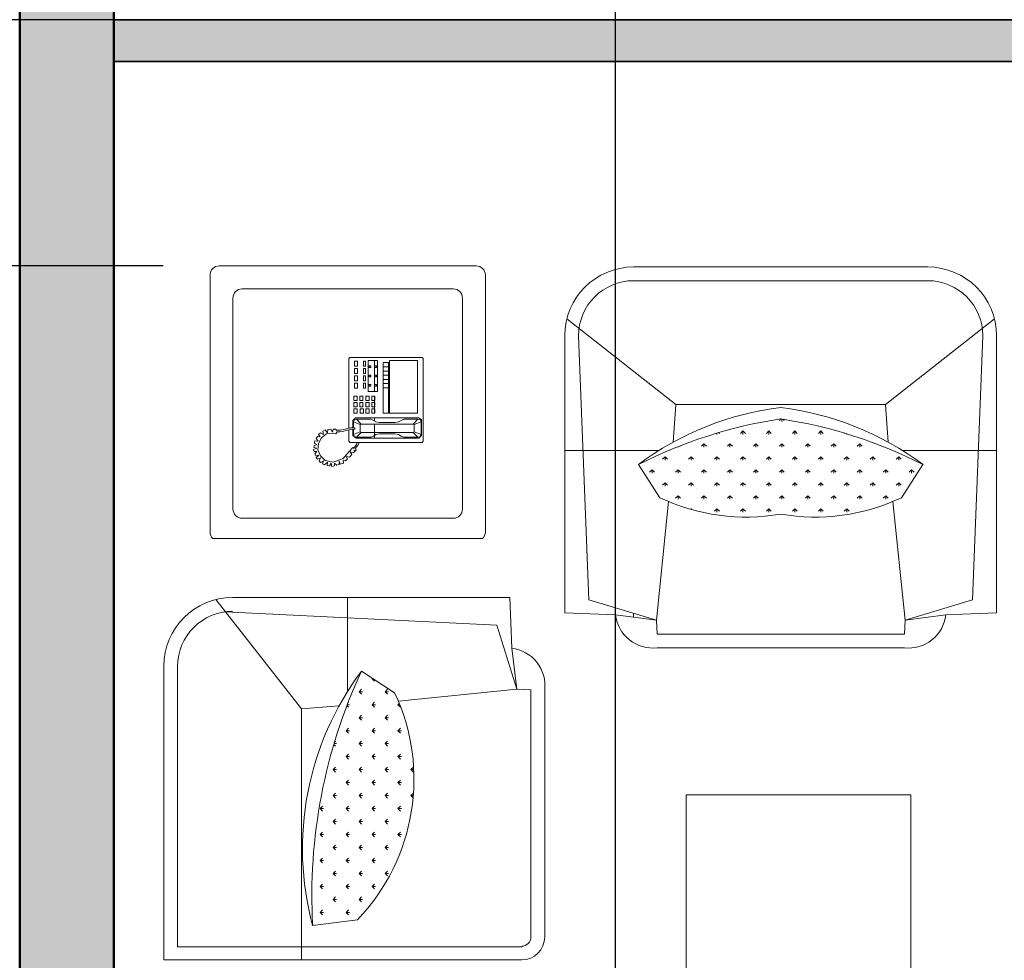
# Model space of a CAD drawing. Units: inches. Extents: x 2796 to 3603, y 978 to 1787.
# Tile 4 of 15: x 3070 to 3165, y 1222 to 1312. Entities that reach past the tile are written whole.
import ezdxf

# ---------------------------------------------------------------- set-up
doc = ezdxf.new("R2010")
doc.units = ezdxf.units.IN
for name, color, linetype, lineweight in [('A-ANNO-DIMS', 7, 'Continuous', 18), ('A-WALL-EXTR-PATT', 1, 'Continuous', 13), ('A-WALL-INTR-PATT', 5, 'Continuous', 13), ('Furniture', 2, 'Continuous', 18), ('Inner Wall', 5, 'Continuous', 35), ('Outer Wall', 1, 'Continuous', 50)]:
    doc.layers.add(name, color=color, linetype=linetype, lineweight=lineweight)
doc.styles.get("Standard").update_dxf_attribs({"font": 'arial.ttf'})
doc.dimstyles.get("Standard").update_dxf_attribs({"dimtxt": 18, "dimasz": 12, "dimexe": 0.18, "dimexo": 0.0625, "dimgap": 0.09, "dimtad": 0, "dimtih": 1, "dimtoh": 1, "dimdec": 0, "dimzin": 0, "dimdsep": 46, "dimlunit": 3, "dimtxsty": 'Standard', "dimcen": 0.09, "dimadec": 0, "dimazin": 0, "dimtfac": 1, "dimtdec": 0, "dimtofl": 0, "dimtmove": 0, "dimatfit": 3, "dimfxl": 1, "dimtolj": 1, "dimtzin": 0, "dimarcsym": 0})

# ---------------------------------------------------------------- blocks, each defined once
blk = doc.blocks.new('A$C16A87060')
at = {"ltscale": 2}
for p, q in [((272, 1415.3), (103.9, 1629.3)), ((362, 1633.4), (362, 1448.5)), ((137, 1606.4), (655.3, 1586)), ((655.3, 1586), (694.6, 1453.8)), ((684.3, 1533.8), (694.6, 1453.8)), ((29, 1498.4), (29, 1209.9)), ((389.7, 1489), (454.7, 1446.7)), ((694.6, 1453.8), (462.1, 1430.1)), ((722, 1452.4), (694.6, 1453.8)), ((722, 1209.9), (722, 1452.4)), ((345.9, 1421), (272, 1415.3)), ((272, 1415.3), (272, 1209.9)), ((29, 921.4), (29, 1209.9)), ((272, 1004.5), (272, 1209.9)), ((722, 1209.9), (722, 967.4)), ((272, 1004.5), (103.9, 790.5)), ((345.9, 998.8), (272, 1004.5)), ((694.6, 966), (462.1, 989.7)), ((362, 786.4), (362, 971.3)), ((389.7, 930.8), (454.7, 973.1)), ((655.3, 833.8), (694.6, 966)), ((684.3, 886), (694.6, 966)), ((722, 967.4), (694.6, 966)), ((137, 813.4), (655.3, 833.8))]:
    blk.add_line(p, q, dxfattribs=at)
for p, q in [((680.7, 1633.4), (137, 1633.4)), ((684.3, 1533.8), (680.7, 1633.4)), ((2, 1498.4), (2, 1209.9)), ((749, 1209.9), (749, 1452.4)), ((1037.3, 1465.2), (2216.9, 1465.2)), ((1037.3, 1024.2), (1037.3, 1465.2)), ((2, 921.4), (2, 1209.9)), ((749, 1209.9), (749, 967.4)), ((2216.9, 1024.2), (1037.3, 1024.2)), ((681.3, 921.3), (688.8, 921.3)), ((684.3, 886), (680.7, 786.4)), ((680.7, 786.4), (137, 786.4)), ((1316.4, 747), (831.4, 747)), ((831.4, 720), (830, 692.5)), ((1316.4, 720), (831.4, 720)), ((1335.7, 27), (1335.7, 702.9)), ((1361.4, 702), (1361.4, 0)), ((750, 682.3), (650.4, 678.6)), ((650.4, 678.6), (650.4, 135)), ((704.4, 653.3), (830, 692.5)), ((750, 682.3), (830, 692.5)), ((830, 692.5), (853.7, 460)), ((678.3, 120.6), (704.4, 653.3)), ((18, 630.6), (522, 630.6)), ((534.7, 625.3), (534.7, 95.9)), ((0, 108.6), (0, 612.6)), ((63, 585.6), (477, 585.6)), ((45, 153.6), (45, 567.6)), ((495, 567.6), (495, 153.6)), ((794.8, 387.7), (837.1, 452.7)), ((185.6, 413.3), (246.3, 413.3)), ((255.5, 413.3), (288.5, 413.3)), ((297.7, 413.3), (304.3, 413.3)), ((310.1, 413.3), (332.3, 413.3)), ((332.3, 413.3), (337.8, 413.3)), ((1282.5, 379.8), (1294.1, 291.9)), ((650.4, 360), (835.3, 360)), ((862.8, 343.9), (868.5, 270)), ((868.5, 270), (654.5, 101.9)), ((868.5, 270), (1361.4, 270)), ((477, 135.6), (63, 135.6)), ((522, 90.6), (18, 90.6)), ((785.4, 27), (1335.7, 27)), ((785.4, 0), (1361.4, 0))]:
    blk.add_line(p, q)
at = {"linetype": 'ByBlock'}
for p, q in [((400, 1466.7), (404.7, 1471.5)), ((400, 1466.7), (406.7, 1466.7)), ((400, 1466.7), (404.7, 1462)), ((374.5, 1441.3), (379.3, 1446.1)), ((374.5, 1441.3), (381.3, 1441.3)), ((374.5, 1441.3), (379.3, 1436.5)), ((425.4, 1441.3), (430.2, 1446.1)), ((425.4, 1441.3), (432.2, 1441.3)), ((425.4, 1441.3), (430.2, 1436.5)), ((400, 1415.8), (404.7, 1420.6)), ((400, 1415.8), (406.7, 1415.8)), ((400, 1415.8), (404.7, 1411.1)), ((450.9, 1415.8), (455.7, 1420.6)), ((450.9, 1415.8), (457.6, 1415.8)), ((450.9, 1415.8), (455.7, 1411.1)), ((374.5, 1390.4), (379.3, 1395.1)), ((425.4, 1390.4), (430.2, 1395.1)), ((374.5, 1390.4), (381.3, 1390.4)), ((374.5, 1390.4), (379.3, 1385.6)), ((425.4, 1390.4), (432.2, 1390.4)), ((425.4, 1390.4), (430.2, 1385.6)), ((349.1, 1364.9), (353.8, 1369.7)), ((349.1, 1364.9), (355.8, 1364.9)), ((349.1, 1364.9), (353.8, 1360.1)), ((400, 1364.9), (404.7, 1369.7)), ((400, 1364.9), (406.7, 1364.9)), ((400, 1364.9), (404.7, 1360.1)), ((450.9, 1364.9), (455.7, 1369.7)), ((450.9, 1364.9), (457.6, 1364.9)), ((450.9, 1364.9), (455.7, 1360.1)), ((328, 1335.1), (328.4, 1334.7)), ((329.3, 1339.5), (330.4, 1339.5)), ((374.5, 1339.5), (379.3, 1344.2)), ((374.5, 1339.5), (381.3, 1339.5)), ((374.5, 1339.5), (379.3, 1334.7)), ((425.4, 1339.5), (430.2, 1344.2)), ((425.4, 1339.5), (432.2, 1339.5)), ((425.4, 1339.5), (430.2, 1334.7)), ((476.3, 1339.5), (481.1, 1344.2)), ((476.3, 1339.5), (483.1, 1339.5)), ((476.3, 1339.5), (481.1, 1334.7)), ((349.1, 1314), (353.8, 1318.8)), ((349.1, 1314), (355.8, 1314)), ((349.1, 1314), (353.8, 1309.2)), ((400, 1314), (404.7, 1318.8)), ((400, 1314), (406.7, 1314)), ((400, 1314), (404.7, 1309.2)), ((450.9, 1314), (455.7, 1318.8)), ((450.9, 1314), (457.6, 1314)), ((450.9, 1314), (455.7, 1309.2)), ((323.6, 1288.5), (328.4, 1293.3)), ((323.6, 1288.5), (330.4, 1288.5)), ((323.6, 1288.5), (328.4, 1283.8)), ((374.5, 1288.5), (379.3, 1293.3)), ((374.5, 1288.5), (381.3, 1288.5)), ((374.5, 1288.5), (379.3, 1283.8)), ((425.4, 1288.5), (430.2, 1293.3)), ((425.4, 1288.5), (432.2, 1288.5)), ((425.4, 1288.5), (430.2, 1283.8)), ((476.3, 1288.5), (481.1, 1293.3)), ((476.3, 1288.5), (483.1, 1288.5)), ((476.3, 1288.5), (481.1, 1283.8)), ((349.1, 1263.1), (353.8, 1267.9)), ((349.1, 1263.1), (355.8, 1263.1)), ((349.1, 1263.1), (353.8, 1258.3)), ((400, 1263.1), (404.7, 1267.9)), ((400, 1263.1), (406.7, 1263.1)), ((400, 1263.1), (404.7, 1258.3)), ((450.9, 1263.1), (455.7, 1267.9)), ((450.9, 1263.1), (457.6, 1263.1)), ((450.9, 1263.1), (455.7, 1258.3)), ((323.6, 1237.6), (328.4, 1242.4)), ((323.6, 1237.6), (330.4, 1237.6)), ((323.6, 1237.6), (328.4, 1232.9)), ((374.5, 1237.6), (379.3, 1242.4)), ((374.5, 1237.6), (381.3, 1237.6)), ((374.5, 1237.6), (379.3, 1232.9)), ((425.4, 1237.6), (430.2, 1242.4)), ((425.4, 1237.6), (432.2, 1237.6)), ((425.4, 1237.6), (430.2, 1232.9)), ((476.3, 1237.6), (481.1, 1242.4)), ((476.3, 1237.6), (483.1, 1237.6)), ((476.3, 1237.6), (481.1, 1232.9)), ((300.8, 1214.8), (302.9, 1216.9)), ((349.1, 1212.2), (353.8, 1216.9)), ((400, 1212.2), (404.7, 1216.9)), ((450.9, 1212.2), (455.7, 1216.9)), ((300.1, 1210.2), (302.9, 1207.4)), ((300.4, 1212.2), (304.9, 1212.2)), ((349.1, 1212.2), (355.8, 1212.2)), ((349.1, 1212.2), (353.8, 1207.4)), ((400, 1212.2), (406.7, 1212.2)), ((400, 1212.2), (404.7, 1207.4)), ((450.9, 1212.2), (457.6, 1212.2)), ((450.9, 1212.2), (455.7, 1207.4)), ((323.6, 1186.7), (328.4, 1191.5)), ((323.6, 1186.7), (330.4, 1186.7)), ((323.6, 1186.7), (328.4, 1181.9)), ((374.5, 1186.7), (379.3, 1191.5)), ((374.5, 1186.7), (381.3, 1186.7)), ((374.5, 1186.7), (379.3, 1181.9)), ((425.4, 1186.7), (430.2, 1191.5)), ((425.4, 1186.7), (432.2, 1186.7)), ((425.4, 1186.7), (430.2, 1181.9)), ((476.3, 1186.7), (481.1, 1191.5)), ((476.3, 1186.7), (483.1, 1186.7)), ((476.3, 1186.7), (481.1, 1181.9)), ((349.1, 1161.3), (353.8, 1166)), ((349.1, 1161.3), (355.8, 1161.3)), ((349.1, 1161.3), (353.8, 1156.5)), ((400, 1161.3), (404.7, 1166)), ((400, 1161.3), (406.7, 1161.3)), ((400, 1161.3), (404.7, 1156.5)), ((450.9, 1161.3), (455.7, 1166)), ((450.9, 1161.3), (457.6, 1161.3)), ((450.9, 1161.3), (455.7, 1156.5)), ((323.6, 1135.8), (328.4, 1140.6)), ((374.5, 1135.8), (379.3, 1140.6)), ((425.4, 1135.8), (430.2, 1140.6)), ((476.3, 1135.8), (481.1, 1140.6)), ((323.6, 1135.8), (330.4, 1135.8)), ((323.6, 1135.8), (328.4, 1131)), ((374.5, 1135.8), (381.3, 1135.8)), ((374.5, 1135.8), (379.3, 1131)), ((425.4, 1135.8), (432.2, 1135.8)), ((425.4, 1135.8), (430.2, 1131)), ((476.3, 1135.8), (483.1, 1135.8)), ((476.3, 1135.8), (481.1, 1131)), ((349.1, 1110.4), (353.8, 1115.1)), ((349.1, 1110.4), (355.8, 1110.4)), ((349.1, 1110.4), (353.8, 1105.6)), ((400, 1110.4), (404.7, 1115.1)), ((400, 1110.4), (406.7, 1110.4)), ((400, 1110.4), (404.7, 1105.6)), ((450.9, 1110.4), (455.7, 1115.1)), ((450.9, 1110.4), (457.6, 1110.4)), ((450.9, 1110.4), (455.7, 1105.6)), ((327, 1088.2), (328.4, 1089.7)), ((327.9, 1084.9), (330.4, 1084.9)), ((374.5, 1084.9), (379.3, 1089.7)), ((374.5, 1084.9), (381.3, 1084.9)), ((374.5, 1084.9), (379.3, 1080.1)), ((425.4, 1084.9), (430.2, 1089.7)), ((425.4, 1084.9), (432.2, 1084.9)), ((425.4, 1084.9), (430.2, 1080.1)), ((476.3, 1084.9), (481.1, 1089.7)), ((476.3, 1084.9), (483.1, 1084.9)), ((476.3, 1084.9), (481.1, 1080.1)), ((349.1, 1059.4), (353.8, 1064.2)), ((400, 1059.4), (404.7, 1064.2)), ((450.9, 1059.4), (455.7, 1064.2)), ((349.1, 1059.4), (355.8, 1059.4)), ((349.1, 1059.4), (353.8, 1054.7)), ((400, 1059.4), (406.7, 1059.4)), ((400, 1059.4), (404.7, 1054.7)), ((450.9, 1059.4), (457.6, 1059.4)), ((450.9, 1059.4), (455.7, 1054.7)), ((374.5, 1034), (379.3, 1038.8)), ((374.5, 1034), (381.3, 1034)), ((374.5, 1034), (379.3, 1029.2)), ((425.4, 1034), (430.2, 1038.8)), ((425.4, 1034), (432.2, 1034)), ((425.4, 1034), (430.2, 1029.2)), ((476.3, 1034), (478, 1035.6)), ((476.3, 1034), (477.5, 1034)), ((476.3, 1034), (477.2, 1033.1)), ((352.9, 1012.4), (353.8, 1013.3)), ((354.5, 1008.5), (355.8, 1008.5)), ((400, 1008.5), (404.7, 1013.3)), ((400, 1008.5), (406.7, 1008.5)), ((400, 1008.5), (404.7, 1003.8)), ((450.9, 1008.5), (455.7, 1013.3)), ((450.9, 1008.5), (457.6, 1008.5)), ((450.9, 1008.5), (455.7, 1003.8)), ((374.5, 983.1), (379.3, 987.8)), ((425.4, 983.1), (430.2, 987.8)), ((374.5, 983.1), (381.3, 983.1)), ((374.5, 983.1), (379.3, 978.3)), ((425.4, 983.1), (432.2, 983.1)), ((425.4, 983.1), (430.2, 978.3)), ((400, 957.6), (404.7, 962.4)), ((400, 957.6), (406.7, 957.6)), ((400, 957.6), (404.7, 952.8)), ((181.5, 508.6), (179.4, 506.6)), ((179.4, 506.6), (179.4, 364.6)), ((181.5, 508.6), (344, 508.6)), ((297.7, 500.4), (301.8, 505.5)), ((301.8, 502.5), (300.8, 498.3)), ((301.8, 505.5), (332.7, 505.5)), ((306, 504.5), (301.8, 502.5)), ((311.1, 491.1), (306, 504.5)), ((306, 504.5), (330.6, 504.5)), ((325.5, 491.1), (330.6, 504.5)), ((330.6, 504.5), (334.8, 502.5)), ((332.7, 505.5), (337.8, 500.4)), ((334.8, 502.5), (335.8, 498.3)), ((344, 508.6), (346.1, 506.6)), ((346.1, 506.6), (346.1, 364.6)), ((288.5, 497.3), (185.6, 497.3)), ((185.6, 497.3), (185.6, 442.8)), ((288.5, 442.8), (288.5, 497.3)), ((297.7, 375.9), (297.7, 500.4)), ((300.8, 498.3), (300.8, 470.6)), ((300.8, 498.3), (310.1, 489.1)), ((310.1, 489.1), (311.1, 491.1)), ((310.1, 442.8), (310.1, 489.1)), ((325.5, 491.1), (311.1, 491.1)), ((326.5, 489.1), (325.5, 491.1)), ((335.8, 498.3), (326.5, 489.1)), ((326.5, 442.8), (326.5, 489.1)), ((335.8, 498.3), (335.8, 470.6)), ((337.8, 500.4), (337.8, 377)), ((988.1, 484.7), (983.3, 489.5)), ((988.1, 484.7), (988.1, 490.2)), ((988.1, 484.7), (992.8, 489.5)), ((1039, 484.7), (1034.2, 489.5)), ((1039, 484.7), (1039, 489.3)), ((1039, 484.7), (1043.2, 488.9)), ((300.8, 470.6), (302.9, 465.4)), ((302.9, 465.4), (306, 460.3)), ((333.7, 465.4), (330.6, 460.3)), ((335.8, 470.6), (333.7, 465.4)), ((860.8, 459.2), (865.5, 464)), ((911.7, 459.2), (906.9, 464)), ((911.7, 459.2), (911.7, 466)), ((911.7, 459.2), (916.5, 464)), ((962.6, 459.2), (957.8, 464)), ((962.6, 459.2), (962.6, 466)), ((962.6, 459.2), (967.4, 464)), ((1013.5, 459.2), (1008.7, 464)), ((1013.5, 459.2), (1013.5, 466)), ((1013.5, 459.2), (1018.3, 464)), ((1064.4, 459.2), (1059.7, 464)), ((1064.4, 459.2), (1064.4, 466)), ((1064.4, 459.2), (1069.2, 464)), ((1115.3, 459.2), (1110.6, 464)), ((1115.3, 459.2), (1115.3, 466)), ((1115.3, 459.2), (1120.1, 464)), ((306, 460.3), (307, 453.1)), ((307, 453.1), (307, 442.8)), ((330.6, 460.3), (329.6, 453.1)), ((329.6, 453.1), (329.6, 442.8)), ((860.8, 459.2), (858.2, 461.8)), ((860.8, 459.2), (860.8, 462.9)), ((185.6, 442.8), (288.5, 442.8)), ((288.5, 440.7), (189.7, 440.7)), ((189.7, 440.7), (189.7, 430.4)), ((189.7, 430.4), (288.5, 430.4)), ((197.9, 440.7), (197.9, 430.4)), ((206.2, 440.7), (206.2, 430.4)), ((214.4, 440.7), (214.4, 430.4)), ((222.6, 440.7), (222.6, 430.4)), ((230.9, 440.7), (230.9, 430.4)), ((239.1, 440.7), (239.1, 430.4)), ((288.5, 430.4), (288.5, 440.7)), ((307, 423.2), (307, 442.8)), ((310.1, 442.8), (310.1, 387.2)), ((326.5, 442.8), (326.5, 387.2)), ((329.6, 423.2), (329.6, 442.8)), ((835.3, 433.8), (830.5, 438.5)), ((835.3, 433.8), (835.3, 440.5)), ((835.3, 433.8), (840.1, 438.5)), ((886.2, 433.8), (881.5, 438.5)), ((886.2, 433.8), (886.2, 440.5)), ((886.2, 433.8), (891, 438.5)), ((937.1, 433.8), (932.4, 438.5)), ((937.1, 433.8), (937.1, 440.5)), ((937.1, 433.8), (941.9, 438.5)), ((988.1, 433.8), (983.3, 438.5)), ((988.1, 433.8), (988.1, 440.5)), ((988.1, 433.8), (992.8, 438.5)), ((1039, 433.8), (1034.2, 438.5)), ((1039, 433.8), (1039, 440.5)), ((1039, 433.8), (1043.7, 438.5)), ((1089.9, 433.8), (1085.1, 438.5)), ((1089.9, 433.8), (1089.9, 440.5)), ((1089.9, 433.8), (1094.7, 438.5)), ((1140.8, 433.8), (1136, 438.5)), ((1140.8, 433.8), (1140.8, 440.5)), ((1140.8, 433.8), (1145.6, 438.5)), ((1191.7, 433.8), (1186.9, 438.5)), ((1191.7, 433.8), (1191.7, 440.5)), ((1191.7, 433.8), (1196.5, 438.5)), ((246.3, 419.1), (185.6, 419.1)), ((185.6, 419.1), (185.6, 400.6)), ((199, 417.1), (195.9, 417.1)), ((195.9, 417.1), (195.9, 414)), ((195.9, 414), (199, 414)), ((195.9, 405.8), (195.9, 402.7)), ((199, 405.8), (195.9, 405.8)), ((199, 414), (199, 417.1)), ((199, 402.7), (199, 405.8)), ((214.4, 417.1), (214.4, 414)), ((217.5, 417.1), (214.4, 417.1)), ((214.4, 414), (217.5, 414)), ((214.4, 405.8), (214.4, 402.7)), ((217.5, 405.8), (214.4, 405.8)), ((217.5, 414), (217.5, 417.1)), ((217.5, 402.7), (217.5, 405.8)), ((232.9, 417.1), (232.9, 414)), ((236, 417.1), (232.9, 417.1)), ((232.9, 414), (236, 414)), ((232.9, 405.8), (232.9, 402.7)), ((236, 405.8), (232.9, 405.8)), ((236, 414), (236, 417.1)), ((236, 402.7), (236, 405.8)), ((246.3, 400.6), (246.3, 419.1)), ((255.5, 414), (263.8, 414)), ((255.5, 407.8), (255.5, 414)), ((263.8, 407.8), (255.5, 407.8)), ((263.8, 414), (263.8, 407.8)), ((267.9, 414), (276.1, 414)), ((267.9, 407.8), (267.9, 414)), ((276.1, 407.8), (267.9, 407.8)), ((276.1, 414), (276.1, 407.8)), ((280.2, 414), (288.5, 414)), ((280.2, 407.8), (280.2, 414)), ((288.5, 407.8), (280.2, 407.8)), ((288.5, 414), (288.5, 407.8)), ((300.8, 405.8), (302.9, 410.9)), ((300.8, 378), (300.8, 405.8)), ((302.9, 410.9), (306, 416)), ((306, 416), (307, 423.2)), ((330.6, 416), (329.6, 423.2)), ((333.7, 410.9), (330.6, 416)), ((335.8, 405.8), (333.7, 410.9)), ((335.8, 378), (335.8, 405.8)), ((809.9, 408.3), (808.9, 409.3)), ((809.9, 408.3), (814.6, 413.1)), ((809.9, 408.3), (809.9, 410.8)), ((860.8, 408.3), (856, 413.1)), ((860.8, 408.3), (860.8, 415.1)), ((860.8, 408.3), (865.5, 413.1)), ((911.7, 408.3), (906.9, 413.1)), ((911.7, 408.3), (911.7, 415.1)), ((911.7, 408.3), (916.5, 413.1)), ((962.6, 408.3), (957.8, 413.1)), ((962.6, 408.3), (962.6, 415.1)), ((962.6, 408.3), (967.4, 413.1)), ((1013.5, 408.3), (1008.7, 413.1)), ((1013.5, 408.3), (1013.5, 415.1)), ((1013.5, 408.3), (1018.3, 413.1)), ((1064.4, 408.3), (1059.7, 413.1)), ((1064.4, 408.3), (1064.4, 415.1)), ((1064.4, 408.3), (1069.2, 413.1)), ((1115.3, 408.3), (1110.6, 413.1)), ((1115.3, 408.3), (1115.3, 415.1)), ((1115.3, 408.3), (1120.1, 413.1)), ((1166.2, 408.3), (1161.5, 413.1)), ((1166.2, 408.3), (1166.2, 415.1)), ((1166.2, 408.3), (1171, 413.1)), ((1217.2, 408.3), (1212.4, 413.1)), ((1217.2, 408.3), (1217.2, 415.1)), ((1217.2, 408.3), (1221.9, 413.1)), ((185.6, 400.6), (246.3, 400.6)), ((196.9, 395.5), (186.6, 395.5)), ((186.6, 395.5), (186.6, 391.4)), ((186.6, 391.4), (196.9, 391.4)), ((195.9, 402.7), (199, 402.7)), ((196.9, 391.4), (196.9, 395.5)), ((211.3, 395.5), (201, 395.5)), ((201, 395.5), (201, 391.4)), ((201, 391.4), (211.3, 391.4)), ((211.3, 391.4), (211.3, 395.5)), ((214.4, 402.7), (217.5, 402.7)), ((215.4, 395.5), (215.4, 391.4)), ((225.7, 395.5), (215.4, 395.5)), ((215.4, 391.4), (225.7, 391.4)), ((225.7, 391.4), (225.7, 395.5)), ((229.8, 395.5), (229.8, 391.4)), ((240.1, 395.5), (229.8, 395.5)), ((229.8, 391.4), (240.1, 391.4)), ((232.9, 402.7), (236, 402.7)), ((240.1, 391.4), (240.1, 395.5)), ((255.5, 402.7), (263.8, 402.7)), ((255.5, 396.5), (255.5, 402.7)), ((263.8, 396.5), (255.5, 396.5)), ((255.5, 390.3), (263.8, 390.3)), ((255.5, 384.2), (255.5, 390.3)), ((263.8, 402.7), (263.8, 396.5)), ((263.8, 390.3), (263.8, 384.2)), ((267.9, 402.7), (276.1, 402.7)), ((267.9, 396.5), (267.9, 402.7)), ((276.1, 396.5), (267.9, 396.5)), ((267.9, 384.2), (267.9, 390.3)), ((267.9, 390.3), (276.1, 390.3)), ((276.1, 402.7), (276.1, 396.5)), ((276.1, 390.3), (276.1, 384.2)), ((280.2, 402.7), (288.5, 402.7)), ((280.2, 396.5), (280.2, 402.7)), ((288.5, 396.5), (280.2, 396.5)), ((280.2, 385.2), (280.2, 391.4)), ((280.2, 391.4), (288.5, 391.4)), ((288.5, 402.7), (288.5, 396.5)), ((288.5, 391.4), (288.5, 385.2)), ((300.8, 378), (310.1, 387.2)), ((310.1, 387.2), (311.1, 385.2)), ((326.5, 387.2), (325.5, 385.2)), ((335.8, 378), (326.5, 387.2)), ((835.3, 382.9), (830.5, 387.6)), ((835.3, 382.9), (835.3, 389.6)), ((835.3, 382.9), (840.1, 387.6)), ((886.2, 382.9), (881.5, 387.6)), ((886.2, 382.9), (886.2, 389.6)), ((886.2, 382.9), (891, 387.6)), ((937.1, 382.9), (932.4, 387.6)), ((937.1, 382.9), (937.1, 389.6)), ((937.1, 382.9), (941.9, 387.6)), ((988.1, 382.9), (983.3, 387.6)), ((988.1, 382.9), (988.1, 389.6)), ((988.1, 382.9), (992.8, 387.6)), ((1039, 382.9), (1034.2, 387.6)), ((1039, 382.9), (1039, 389.6)), ((1039, 382.9), (1043.7, 387.6)), ((1089.9, 382.9), (1085.1, 387.6)), ((1089.9, 382.9), (1089.9, 389.6)), ((1089.9, 382.9), (1094.7, 387.6)), ((1140.8, 382.9), (1136, 387.6)), ((1140.8, 382.9), (1140.8, 389.6)), ((1140.8, 382.9), (1145.6, 387.6)), ((1191.7, 382.9), (1186.9, 387.6)), ((1191.7, 382.9), (1191.7, 389.6)), ((1191.7, 382.9), (1196.5, 387.6)), ((1242.6, 382.9), (1237.8, 387.6)), ((1242.6, 382.9), (1242.6, 389.6)), ((1242.6, 382.9), (1247.4, 387.6)), ((186.6, 380), (196.9, 380)), ((186.6, 373.9), (186.6, 380)), ((196.9, 373.9), (186.6, 373.9)), ((196.9, 380), (196.9, 373.9)), ((201, 380), (211.3, 380)), ((201, 373.9), (201, 380)), ((211.3, 373.9), (201, 373.9)), ((211.3, 380), (211.3, 373.9)), ((215.4, 373.9), (215.4, 380)), ((215.4, 380), (225.7, 380)), ((225.7, 373.9), (215.4, 373.9)), ((225.7, 380), (225.7, 373.9)), ((229.8, 373.9), (229.8, 380)), ((229.8, 380), (240.1, 380)), ((240.1, 373.9), (229.8, 373.9)), ((240.1, 380), (240.1, 373.9)), ((263.8, 384.2), (255.5, 384.2)), ((255.5, 379), (263.8, 379)), ((255.5, 372.8), (255.5, 379)), ((263.8, 372.8), (255.5, 372.8)), ((263.8, 379), (263.8, 372.8)), ((276.1, 384.2), (267.9, 384.2)), ((267.9, 379), (276.1, 379)), ((267.9, 372.8), (267.9, 379)), ((276.1, 372.8), (267.9, 372.8)), ((276.1, 379), (276.1, 372.8)), ((288.5, 385.2), (280.2, 385.2)), ((280.2, 372.8), (280.2, 379)), ((280.2, 379), (288.5, 379)), ((288.5, 372.8), (280.2, 372.8)), ((288.5, 379), (288.5, 372.8)), ((302.9, 370.8), (297.7, 375.9)), ((301.8, 373.9), (300.8, 378)), ((306, 371.8), (301.8, 373.9)), ((317.3, 370.8), (302.9, 370.8)), ((311.1, 385.2), (306, 371.8)), ((306, 371.8), (317.3, 371.8)), ((325.5, 385.2), (311.1, 385.2)), ((320.4, 374.9), (317.3, 374.9)), ((317.3, 374.9), (317.4, 366)), ((321, 366.7), (320.4, 374.9)), ((320.6, 371.8), (330.6, 371.8)), ((332.7, 370.8), (320.7, 370.8)), ((325.5, 385.2), (330.6, 371.8)), ((330.6, 371.8), (334.8, 373.9)), ((337.8, 377), (332.7, 370.8)), ((334.8, 373.9), (335.8, 378)), ((352.2, 380.8), (346.1, 383.1)), ((346.1, 379), (350.6, 377.8)), ((350.6, 377.8), (354.8, 374.5)), ((355.1, 377.9), (352.2, 380.8)), ((354.8, 374.5), (355.9, 373)), ((357.3, 375.9), (355.1, 377.9)), ((358, 373.2), (355.9, 371)), ((355.9, 373), (358, 373.2)), ((355.9, 371), (364.2, 363.6)), ((361.1, 377.4), (357.3, 375.9)), ((362.9, 375.6), (361.1, 377.4)), ((361.5, 372.5), (362.9, 375.6)), ((364, 374.5), (361.5, 372.5)), ((366.7, 371.6), (364, 374.5)), ((364.6, 365.6), (366.7, 371.6)), ((370.2, 368.5), (364.6, 365.6)), ((374.9, 364), (370.2, 368.5)), ((179.4, 364.6), (181.5, 362.6)), ((318.2, 362.6), (181.5, 362.6)), ((317.4, 366), (319.9, 355.6)), ((319.9, 355.6), (322.4, 345.8)), ((322.4, 360), (321, 366.7)), ((344, 362.6), (321.8, 362.6)), ((324.9, 350.2), (322.4, 360)), ((325.5, 345.2), (324.9, 350.2)), ((346.1, 364.6), (344, 362.6)), ((364.2, 363.6), (377.8, 352)), ((373.8, 357.4), (374.9, 364)), ((378.5, 360.3), (373.8, 357.4)), ((378, 351.7), (384.9, 332.1)), ((382.5, 356.2), (378.5, 360.3)), ((380.9, 351.6), (382.5, 356.2)), ((387.2, 352.3), (380.9, 351.7)), ((389, 346), (387.2, 352.3)), ((857, 361.2), (856, 362.2)), ((860.8, 359.7), (860.8, 364.2)), ((862.5, 359.1), (865.5, 362.2)), ((911.7, 357.4), (906.9, 362.2)), ((911.7, 357.4), (911.7, 364.2)), ((911.7, 357.4), (916.5, 362.2)), ((962.6, 357.4), (957.8, 362.2)), ((962.6, 357.4), (962.6, 364.2)), ((962.6, 357.4), (967.4, 362.2)), ((1013.5, 357.4), (1008.7, 362.2)), ((1013.5, 357.4), (1013.5, 364.2)), ((1013.5, 357.4), (1018.3, 362.2)), ((1064.4, 357.4), (1059.7, 362.2)), ((1064.4, 357.4), (1064.4, 364.2)), ((1064.4, 357.4), (1069.2, 362.2)), ((1115.3, 357.4), (1110.6, 362.2)), ((1115.3, 357.4), (1115.3, 364.2)), ((1115.3, 357.4), (1120.1, 362.2)), ((1166.2, 357.4), (1161.5, 362.2)), ((1166.2, 357.4), (1166.2, 364.2)), ((1166.2, 357.4), (1171, 362.2)), ((1217.2, 357.4), (1212.4, 362.2)), ((1217.2, 357.4), (1217.2, 364.2)), ((1217.2, 357.4), (1221.9, 362.2)), ((1268.1, 357.4), (1263.3, 362.2)), ((1268.1, 357.4), (1268.1, 364.2)), ((1268.1, 357.4), (1272.8, 362.2)), ((320.5, 336.9), (320.1, 331.9)), ((320.1, 331.9), (326.2, 330.8)), ((326.2, 330.8), (320.3, 327.3)), ((322.8, 339.2), (320.5, 336.9)), ((322.4, 345.8), (322.2, 340.4)), ((322.2, 340.4), (322.8, 339.2)), ((325.3, 339.8), (325.5, 345.2)), ((329.1, 337.1), (325.3, 339.8)), ((328.2, 332.3), (329.1, 337.1)), ((329.3, 319.2), (328.2, 332.3)), ((384.9, 332.1), (381.9, 316.5)), ((383, 343.7), (389, 346)), ((389.7, 343.9), (383, 343.7)), ((386.7, 335), (391.1, 339.2)), ((392.4, 335), (386.7, 335)), ((386.9, 327.9), (393.4, 329.8)), ((391.1, 339.2), (389.7, 343.9)), ((393.4, 329.8), (392.4, 335)), ((934.6, 334.5), (932.4, 336.7)), ((937.1, 333.7), (937.1, 338.7)), ((938.5, 333.3), (941.9, 336.7)), ((988.1, 331.9), (983.3, 336.7)), ((988.1, 331.9), (988.1, 338.7)), ((988.1, 331.9), (992.8, 336.7)), ((1039, 331.9), (1034.2, 336.7)), ((1039, 331.9), (1039, 338.7)), ((1039, 331.9), (1043.7, 336.7)), ((1089.9, 331.9), (1085.1, 336.7)), ((1089.9, 331.9), (1089.9, 338.7)), ((1089.9, 331.9), (1094.7, 336.7)), ((1140.8, 331.9), (1136, 336.7)), ((1140.8, 331.9), (1140.8, 338.7)), ((1140.8, 331.9), (1145.6, 336.7)), ((1191.7, 331.9), (1186.9, 336.7)), ((1191.7, 331.9), (1191.7, 338.7)), ((1191.7, 331.9), (1196.5, 336.7)), ((1242.6, 331.9), (1237.8, 336.7)), ((1242.6, 331.9), (1242.6, 338.7)), ((1242.6, 331.9), (1247.4, 336.7)), ((320.3, 327.3), (320.7, 321.7)), ((320.7, 321.7), (327.4, 321)), ((327.4, 321), (321.6, 316.5)), ((321.6, 316.5), (324.3, 311.7)), ((324.3, 311.7), (330.5, 312.9)), ((330.5, 312.9), (327.6, 307.1)), ((337.2, 309.2), (329.3, 319.2)), ((348.2, 303.3), (337.2, 309.2)), ((381.9, 316.5), (372.8, 307.5)), ((385.3, 307.3), (382.4, 312.9)), ((382.4, 312.9), (388.4, 311)), ((385.1, 320.8), (391.5, 320.6)), ((390.1, 315.2), (385.1, 320.8)), ((392.4, 324.8), (386.9, 327.9)), ((388.4, 311), (390.1, 315.2)), ((391.5, 320.6), (392.4, 324.8)), ((1064.4, 306.5), (1059.7, 311.3)), ((1064.4, 306.5), (1064.4, 313.2)), ((1064.4, 306.5), (1069.2, 311.3)), ((1115.3, 306.5), (1110.6, 311.3)), ((1115.3, 306.5), (1115.3, 313.2)), ((1115.3, 306.5), (1120.1, 311.3)), ((1166.2, 306.5), (1161.5, 311.3)), ((1166.2, 306.5), (1166.2, 313.2)), ((1166.2, 306.5), (1171, 311.3)), ((1217.2, 306.5), (1212.4, 311.3)), ((1217.2, 306.5), (1217.2, 313.2)), ((1217.2, 306.5), (1221.9, 311.3)), ((1268.1, 306.5), (1263.3, 311.3)), ((1268.1, 306.5), (1268.1, 313.2)), ((1268.1, 306.5), (1272.8, 311.3)), ((327.6, 307.1), (330.7, 303.3)), ((330.7, 303.3), (335.5, 306.9)), ((335.5, 306.9), (334.7, 301.2)), ((334.7, 301.2), (338.6, 298.7)), ((338.6, 298.7), (343.6, 302.9)), ((343.6, 302.9), (343, 296)), ((343, 296), (347.4, 294.8)), ((347.4, 294.8), (350.1, 300.4)), ((360.7, 302.3), (348.2, 303.3)), ((350.1, 300.4), (352.6, 294.8)), ((352.6, 294.8), (356.1, 294.4)), ((356.1, 294.4), (357.6, 300.4)), ((357.6, 300.4), (359.9, 293.7)), ((359.9, 293.7), (363.8, 294.8)), ((372.8, 307.5), (360.7, 302.3)), ((363.8, 294.8), (364, 300.4)), ((364, 300.4), (368.8, 296.2)), ((368.8, 296.2), (372.2, 297.9)), ((371.5, 304.2), (375.9, 298.7)), ((372.2, 297.9), (371.5, 304.2)), ((375.9, 298.7), (379.2, 301.7)), ((376.7, 307.3), (382.6, 304.8)), ((379.2, 301.7), (376.7, 307.3)), ((382.6, 304.8), (385.3, 307.3))]:
    blk.add_line(p, q, dxfattribs=at)
for centre, radius, start, end in [((137, 1498.4), 135, 90, 180), ((676.1, 1460.8), 73.4, 353.4179, 83.5749), ((676.1, 959), 73.4, 276.4251, 6.5821), ((137, 921.4), 135, 180, 270), ((823, 674.1), 73.4, 83.4179, 173.5749), ((1316.4, 702), 45, 0, 90), ((1316.4, 702), 18, 0, 90), ((18, 612.6), 18, 90, 180), ((522, 612.6), 18, 45, 90), ((63, 567.6), 18, 90, 180), ((477, 567.6), 18, 0, 90), ((1006.8, 92.3), 398.3, 46.1942, 115.2134), ((1142.9, 853.2), 581.3, 233.2071, 285.072), ((1235.6, 1336.1), 1045.8, 245.0725, 273.2065), ((63, 153.6), 18, 180, 270), ((477, 153.6), 18, 270, 0), ((785.4, 135), 135, 180, 270), ((785.4, 135), 108, 180, 270), ((18, 108.6), 18, 180, 270), ((522, 108.6), 18, 270, 315)]:
    blk.add_arc(centre, radius, start, end)
at = {"ltscale": 2}
for centre, radius, start, end in [((137, 1498.4), 108, 90, 180), ((855.2, 1140.9), 581.3, 143.2071, 173.1788), ((1200, 1074.7), 910, 152.9196, 171.457), ((94.3, 1277), 398.3, 350.3046, 25.2134), ((855.2, 1278.9), 581.3, 186.8212, 216.7929), ((1200, 1345.1), 910, 188.543, 207.0804), ((94.3, 1142.8), 398.3, 334.7866, 9.6954), ((137, 921.4), 108, 180, 270)]:
    blk.add_arc(centre, radius, start, end, dxfattribs=at)
blk = doc.blocks.new('*D12')
at = {"layer": 'A-ANNO-DIMS', "color": 0, "lineweight": -2, "transparency": 16777216}
for p, q in [((3070.183, 1736.675), (3041.33, 1736.675)), ((3041.51, 1724.675), (3041.51, 1391.956)), ((3041.51, 1040.675), (3041.51, 1373.395)), ((3070.183, 1028.675), (3041.33, 1028.675))]:
    blk.add_line(p, q, dxfattribs=at)
at = {"layer": 'A-ANNO-DIMS', "color": 0, "transparency": 16777216}
for points in [[(3039.51, 1724.675), (3043.51, 1724.675), (3041.51, 1736.675)], [(3039.51, 1040.675), (3043.51, 1040.675), (3041.51, 1028.675)]]:
    blk.add_solid(points, dxfattribs=at)
at = {"layer": 'Defpoints', "color": 0, "transparency": 16777216}
for p in [(3041.51, 1736.675), (3070.245, 1736.675), (3070.245, 1028.675)]:
    blk.add_point(p, dxfattribs=at)
at = {"layer": 'A-ANNO-DIMS', "color": 0, "transparency": 16777216, "insert": (3041.51, 1382.675), "char_height": 18, "attachment_point": 5}
blk.add_mtext("\\A1;59'", dxfattribs=at)
blk = doc.blocks.new('*D30')
at = {"layer": 'A-ANNO-DIMS', "color": 0, "lineweight": -2, "transparency": 16777216}
for p, q in [((3083.983, 1288.1), (3059.973, 1288.1)), ((3060.153, 1276.1), (3060.153, 1217.865)), ((3060.153, 1140.812), (3060.153, 1199.046)), ((3083.983, 1128.812), (3059.973, 1128.812))]:
    blk.add_line(p, q, dxfattribs=at)
at = {"layer": 'A-ANNO-DIMS', "color": 0, "transparency": 16777216}
for points in [[(3058.153, 1276.1), (3062.153, 1276.1), (3060.153, 1288.1)], [(3058.153, 1140.812), (3062.153, 1140.812), (3060.153, 1128.812)]]:
    blk.add_solid(points, dxfattribs=at)
at = {"layer": 'Defpoints', "color": 0, "transparency": 16777216}
for p in [(3084.046, 1288.1), (3060.153, 1128.812), (3084.046, 1128.812)]:
    blk.add_point(p, dxfattribs=at)
at = {"layer": 'A-ANNO-DIMS', "color": 0, "transparency": 16777216, "insert": (3060.153, 1208.456), "char_height": 18, "attachment_point": 5}
blk.add_mtext('\\A1;SEATING GROUP 13\'-3 1/2"', dxfattribs=at)
blk = doc.blocks.new('*D51')
at = {"layer": 'A-ANNO-DIMS', "color": 0, "lineweight": -2, "transparency": 16777216}
for p, q in [((3127.245499, 1431.61284), (3127.245499, 989.79534)), ((3199.245499, 1431.61284), (3199.245499, 989.79534)), ((3115.245499, 989.97534), (3103.245499, 989.97534)), ((3211.245499, 989.97534), (3223.245499, 989.97534))]:
    blk.add_line(p, q, dxfattribs=at)
at = {"layer": 'A-ANNO-DIMS', "color": 0, "transparency": 16777216}
for points in [[(3115.245499, 991.97534), (3115.245499, 987.97534), (3127.245499, 989.97534)], [(3211.245499, 991.97534), (3211.245499, 987.97534), (3199.245499, 989.97534)]]:
    blk.add_solid(points, dxfattribs=at)
at = {"layer": 'Defpoints', "color": 0, "transparency": 16777216}
for p in [(3127.245499, 1431.67534), (3199.245499, 1431.67534), (3199.245499, 989.97534)]:
    blk.add_point(p, dxfattribs=at)
at = {"layer": 'A-ANNO-DIMS', "color": 0, "transparency": 16777216, "insert": (3163.245499, 989.97534), "char_height": 18, "attachment_point": 5}
blk.add_mtext('\\A1;6\'-0"', dxfattribs=at)
blk = doc.blocks.new('*D53')
at = {"layer": 'A-ANNO-DIMS', "color": 0, "lineweight": -2, "transparency": 16777216}
for p, q in [((3031.545499, 1347.67534), (3031.545499, 1359.67534)), ((3333.182999, 1335.67534), (3031.365499, 1335.67534)), ((3333.182999, 1311.67534), (3031.365499, 1311.67534)), ((3031.545499, 1299.67534), (3031.545499, 1287.67534))]:
    blk.add_line(p, q, dxfattribs=at)
at = {"layer": 'A-ANNO-DIMS', "color": 0, "transparency": 16777216}
for points in [[(3029.545499, 1347.67534), (3033.545499, 1347.67534), (3031.545499, 1335.67534)], [(3029.545499, 1299.67534), (3033.545499, 1299.67534), (3031.545499, 1311.67534)]]:
    blk.add_solid(points, dxfattribs=at)
at = {"layer": 'Defpoints', "color": 0, "transparency": 16777216}
for p in [(3031.545499, 1335.67534), (3333.245499, 1335.67534), (3333.245499, 1311.67534)]:
    blk.add_point(p, dxfattribs=at)
at = {"layer": 'A-ANNO-DIMS', "color": 0, "transparency": 16777216, "insert": (3031.545499, 1323.67534), "char_height": 18, "attachment_point": 5}
blk.add_mtext('\\A1;2\'-0"', dxfattribs=at)

msp = doc.modelspace()

# ---------------------------------------------------------------- hatches: boundary and pattern name
at = {"layer": 'A-WALL-EXTR-PATT'}
h = msp.add_hatch(color=256, dxfattribs=at)
h.dxf.hatch_style = 1
h.paths.add_polyline_path([(3424.245, 1736.675), (3070.245, 1736.675), (3070.245, 1106.675), (3227.245, 1106.675), (3227.245, 1115.675), (3226.745, 1115.675), (3223.745, 1115.675), (3079.245, 1115.675), (3079.245, 1727.675), (3127.245, 1727.675), (3415.245, 1727.675), (3415.245, 1188.675), (3424.245, 1188.675)])
h.paths.add_polyline_path([(3291.245, 1032.675), (3074.245, 1032.675), (3074.245, 1106.675), (3070.245, 1106.675), (3070.245, 1028.675), (3291.245, 1028.675)])
h.paths.add_polyline_path([(3291.245, 1115.675), (3281.245, 1115.675), (3281.245, 1106.675), (3291.245, 1106.675)], flags=17)
h.paths.add_polyline_path([(3301.245, 1037.675), (3291.245, 1037.675), (3291.245, 1028.675), (3301.245, 1028.675)])
h.paths.add_polyline_path([(3424.245, 1037.675), (3414.245, 1037.675), (3414.245, 1028.675), (3424.245, 1028.675)])
h.paths.add_polyline_path([(3424.245, 1188.675), (3420.245, 1188.675), (3420.245, 1037.675), (3424.245, 1037.675)])
at = {"layer": 'A-WALL-INTR-PATT'}
h = msp.add_hatch(color=256, dxfattribs=at)
h.dxf.hatch_style = 1
h.paths.add_polyline_path([(3249.245, 1727.675), (3245.245, 1727.675), (3245.245, 1655.675), (3103.245, 1655.675), (3103.245, 1651.675), (3245.245, 1651.675), (3245.245, 1503.675), (3249.245, 1503.675)])
h.paths.add_polyline_path([(3131.245, 1727.675), (3127.245, 1727.675), (3127.245, 1703.675), (3127.245, 1679.675), (3131.245, 1679.675)], flags=17)
h.paths.add_polyline_path([(3391.245, 1655.675), (3325.245, 1655.675), (3325.245, 1727.675), (3321.245, 1727.675), (3321.245, 1655.675), (3273.245, 1655.675), (3273.245, 1651.675), (3391.245, 1651.675)])
h.paths.add_polyline_path([(3203.245, 1459.675), (3079.245, 1459.675), (3079.245, 1455.675), (3199.245, 1455.675), (3199.245, 1431.675), (3199.245, 1347.675), (3203.245, 1347.675)])
h.paths.add_polyline_path([(3209.245, 1507.675), (3079.245, 1507.675), (3079.245, 1503.675), (3209.245, 1503.675)])
h.paths.add_polyline_path([(3415.245, 1507.675), (3285.245, 1507.675), (3285.245, 1503.675), (3415.245, 1503.675)])
h.paths.add_polyline_path([(3415.245, 1459.675), (3333.245, 1459.675), (3333.245, 1455.675), (3415.245, 1455.675)])
h.paths.add_polyline_path([(3291.245, 1311.675), (3287.245, 1311.675), (3287.245, 1192.675), (3227.245, 1192.675), (3227.245, 1267.675), (3263.245, 1267.675), (3263.245, 1271.675), (3223.245, 1271.675), (3223.245, 1151.675), (3227.245, 1151.675), (3227.245, 1188.675), (3291.245, 1188.675)])
h.paths.add_polyline_path([(3227.245, 1311.675), (3079.245, 1311.675), (3079.245, 1307.675), (3227.245, 1307.675)])

# ---------------------------------------------------------------- linework, layer by layer
at = {"layer": 'Inner Wall'}
for p, q in [((3079.245, 1311.675), (3227.245, 1311.675)), ((3079.245, 1307.675), (3227.245, 1307.675))]:
    msp.add_line(p, q, dxfattribs=at)
at = {"layer": 'Outer Wall'}
for p, q in [((3070.245, 1028.675), (3070.245, 1736.675)), ((3079.245, 1115.675), (3079.245, 1727.675))]:
    msp.add_line(p, q, dxfattribs=at)

# ---------------------------------------------------------------- block references
at = {"layer": 'Furniture', "xscale": 0.0488098627676315, "yscale": 0.0488098627676315, "zscale": 0.0488098627676315, "rotation": 270}
msp.add_blockref('A$C16A87060', (3084.046, 1288.1), dxfattribs=at)

# ---------------------------------------------------------------- dimensions: what is measured, and where the dimension line sits
at = {"layer": 'A-ANNO-DIMS'}
for base, p1, p2, override, picture, middle in [((3041.51, 1736.675), (3070.245, 1028.675), (3070.245, 1736.675), {"dimclrd": 0, "dimclre": 0, "dimclrt": 0}, '*D12', (3041.51, 1382.675)), ((3031.545, 1335.675), (3333.245, 1311.675), (3333.245, 1335.675), {"dimdec": 1, "dimlfac": 1, "dimrnd": 0, "dimzin": 1, "dimdsep": 46, "dimlunit": 4, "dimfrac": 2}, '*D53', (3031.545, 1323.675))]:
    dim = msp.add_linear_dim(base=base, p1=p1, p2=p2, angle=90, dimstyle='Standard', override=override, dxfattribs=at)
    dim.commit()
    dim.dimension.update_dxf_attribs({"geometry": picture, "text_midpoint": middle})
dim = msp.add_linear_dim(base=(3199.245, 989.975), p1=(3127.245, 1431.675), p2=(3199.245, 1431.675), dimstyle='Standard', override={"dimdec": 1, "dimlfac": 1, "dimrnd": 0, "dimzin": 1, "dimdsep": 46, "dimlunit": 4, "dimfrac": 2}, dxfattribs=at)
dim.commit()
dim.dimension.update_dxf_attribs({"geometry": '*D51', "text_midpoint": (3163.245, 989.975)})
dim = msp.add_linear_dim(base=(3060.153, 1128.812), p1=(3084.046, 1288.1), p2=(3084.046, 1128.812), angle=270, text='SEATING GROUP <>', dimstyle='Standard', override={"dimdec": 1, "dimlfac": 1, "dimrnd": 0, "dimzin": 1, "dimdsep": 46, "dimlunit": 4, "dimfrac": 2}, dxfattribs=at)
dim.commit()
dim.dimension.update_dxf_attribs({"geometry": '*D30', "text_midpoint": (3060.153, 1208.456)})

doc.saveas('drawing.dxf')
